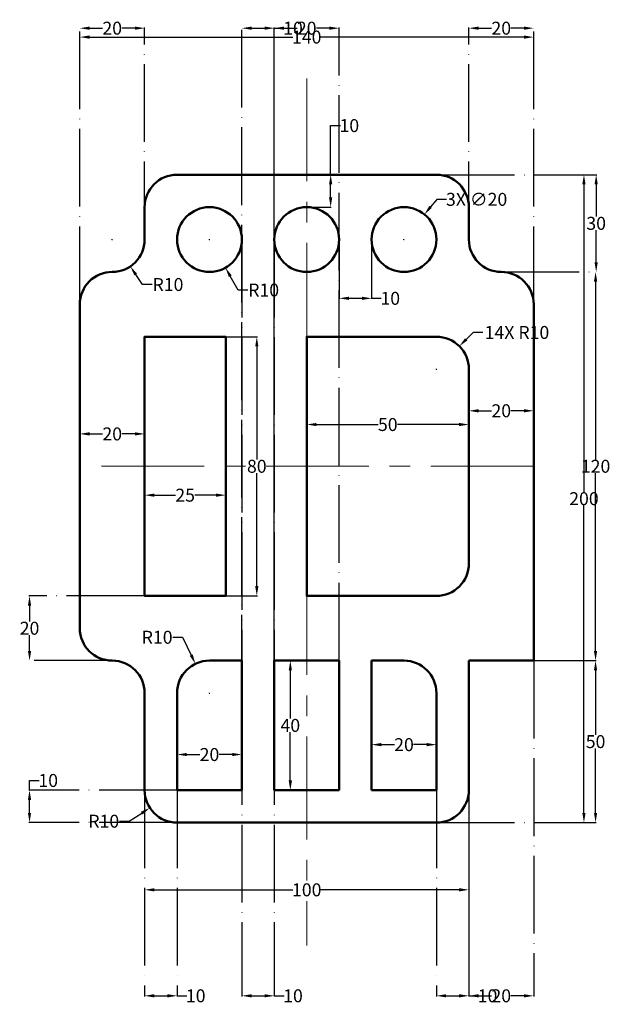
# Model space of a CAD drawing. Units: inches. Extents: x 184 to 366, y 103 to 407.
import ezdxf

# ---------------------------------------------------------------- set-up
doc = ezdxf.new("R2010")
doc.units = ezdxf.units.IN
doc.header["$MEASUREMENT"] = 0
doc.linetypes.add('ACAD_ISO04W100', pattern=[30, 24, -3, 0, -3])
doc.linetypes.add('CENTER', pattern=[50.8, 31.75, -6.35, 6.35, -6.35])
for name, color, linetype, lineweight in [('M-CNTR', 4, 'CENTER', 18), ('M-DIMS', 2, 'Continuous', 25), ('M-OUTL', 7, 'Continuous', 50)]:
    doc.layers.add(name, color=color, linetype=linetype, lineweight=lineweight)
doc.styles.get("Standard").update_dxf_attribs({"font": 'arial.ttf'})
doc.dimstyles.get("Standard").update_dxf_attribs({"dimtxt": 4, "dimasz": 3, "dimexe": 0.18, "dimexo": 0.0625, "dimgap": 0.09, "dimtad": 0, "dimtih": 1, "dimtoh": 1, "dimdec": 0, "dimzin": 0, "dimdsep": 46, "dimtxsty": 'Standard', "dimcen": 0.09, "dimadec": 0, "dimazin": 0, "dimtfac": 1, "dimtdec": 0, "dimtofl": 0, "dimtmove": 0, "dimatfit": 3, "dimfxl": 1, "dimtolj": 1, "dimtzin": 0, "dimarcsym": 0})

# ---------------------------------------------------------------- blocks, each defined once
blk = doc.blocks.new('*D1')
at = {"layer": 'Defpoints', "color": 0, "transparency": 16777216}
for p in [(267.46, 209.15), (267.46, 169.15), (267.46, 169.15)]:
    blk.add_point(p, dxfattribs=at)
at = {"layer": 'M-DIMS', "color": 0, "linetype": 'ACAD_ISO04W100', "lineweight": -2, "transparency": 16777216}
for p, q in [((267.53, 209.15), (267.64, 209.15)), ((267.53, 169.15), (267.64, 169.15))]:
    blk.add_line(p, q, dxfattribs=at)
at = {"layer": 'M-DIMS', "color": 0, "lineweight": -2, "transparency": 16777216}
for p, q in [((267.46, 206.15), (267.46, 191.28)), ((267.46, 172.15), (267.46, 187.02))]:
    blk.add_line(p, q, dxfattribs=at)
at = {"layer": 'M-DIMS', "color": 0, "transparency": 16777216}
for points in [[(266.96, 206.15), (267.96, 206.15), (267.46, 209.15)], [(266.96, 172.15), (267.96, 172.15), (267.46, 169.15)]]:
    blk.add_solid(points, dxfattribs=at)
at = {"layer": 'M-DIMS', "color": 0, "transparency": 16777216, "insert": (267.46, 189.15), "char_height": 4, "attachment_point": 5}
blk.add_mtext('\\A1;40', dxfattribs=at)
blk = doc.blocks.new('*D2')
at = {"layer": 'Defpoints', "color": 0, "transparency": 16777216}
for p in [(232.52, 180.16), (232.52, 180.16), (252.52, 180.16)]:
    blk.add_point(p, dxfattribs=at)
at = {"layer": 'M-DIMS', "color": 0, "linetype": 'ACAD_ISO04W100', "lineweight": -2, "transparency": 16777216}
for p, q in [((232.52, 180.22), (232.52, 180.34)), ((252.52, 180.22), (252.52, 180.34))]:
    blk.add_line(p, q, dxfattribs=at)
at = {"layer": 'M-DIMS', "color": 0, "lineweight": -2, "transparency": 16777216}
for p, q in [((235.52, 180.16), (239.54, 180.16)), ((249.52, 180.16), (245.5, 180.16))]:
    blk.add_line(p, q, dxfattribs=at)
at = {"layer": 'M-DIMS', "color": 0, "transparency": 16777216}
for points in [[(235.52, 180.66), (235.52, 179.66), (232.52, 180.16)], [(249.52, 180.66), (249.52, 179.66), (252.52, 180.16)]]:
    blk.add_solid(points, dxfattribs=at)
at = {"layer": 'M-DIMS', "color": 0, "transparency": 16777216, "insert": (242.52, 180.16), "char_height": 4, "attachment_point": 5}
blk.add_mtext('\\A1;20', dxfattribs=at)
blk = doc.blocks.new('*D3')
at = {"layer": 'Defpoints', "color": 0, "transparency": 16777216}
for p in [(292.52, 183.21), (312.52, 183.21), (312.52, 183.21)]:
    blk.add_point(p, dxfattribs=at)
at = {"layer": 'M-DIMS', "color": 0, "linetype": 'ACAD_ISO04W100', "lineweight": -2, "transparency": 16777216}
for p, q in [((292.52, 183.28), (292.52, 183.39)), ((312.52, 183.28), (312.52, 183.39))]:
    blk.add_line(p, q, dxfattribs=at)
at = {"layer": 'M-DIMS', "color": 0, "lineweight": -2, "transparency": 16777216}
for p, q in [((295.52, 183.21), (299.54, 183.21)), ((309.52, 183.21), (305.5, 183.21))]:
    blk.add_line(p, q, dxfattribs=at)
at = {"layer": 'M-DIMS', "color": 0, "transparency": 16777216}
for points in [[(295.52, 183.71), (295.52, 182.71), (292.52, 183.21)], [(309.52, 183.71), (309.52, 182.71), (312.52, 183.21)]]:
    blk.add_solid(points, dxfattribs=at)
at = {"layer": 'M-DIMS', "color": 0, "transparency": 16777216, "insert": (302.52, 183.21), "char_height": 4, "attachment_point": 5}
blk.add_mtext('\\A1;20', dxfattribs=at)
blk = doc.blocks.new('*D4')
at = {"layer": 'Defpoints', "color": 0, "transparency": 16777216}
for p in [(222.52, 169.15), (322.52, 169.15), (322.52, 138.39)]:
    blk.add_point(p, dxfattribs=at)
at = {"layer": 'M-DIMS', "color": 0, "linetype": 'ACAD_ISO04W100', "lineweight": -2, "transparency": 16777216}
for p, q in [((222.52, 169.09), (222.52, 138.21)), ((322.52, 169.09), (322.52, 138.21))]:
    blk.add_line(p, q, dxfattribs=at)
at = {"layer": 'M-DIMS', "color": 0, "lineweight": -2, "transparency": 16777216}
for p, q in [((225.52, 138.39), (268.2, 138.39)), ((319.52, 138.39), (276.83, 138.39))]:
    blk.add_line(p, q, dxfattribs=at)
at = {"layer": 'M-DIMS', "color": 0, "transparency": 16777216}
for points in [[(225.52, 138.89), (225.52, 137.89), (222.52, 138.39)], [(319.52, 138.89), (319.52, 137.89), (322.52, 138.39)]]:
    blk.add_solid(points, dxfattribs=at)
at = {"layer": 'M-DIMS', "color": 0, "transparency": 16777216, "insert": (272.52, 138.39), "char_height": 4, "attachment_point": 5}
blk.add_mtext('\\A1;100', dxfattribs=at)
blk = doc.blocks.new('*D5')
at = {"layer": 'Defpoints', "color": 0, "transparency": 16777216}
for p in [(272.52, 282.04), (272.52, 269.15), (322.52, 269.15)]:
    blk.add_point(p, dxfattribs=at)
at = {"layer": 'M-DIMS', "color": 0, "linetype": 'ACAD_ISO04W100', "lineweight": -2, "transparency": 16777216}
for p, q in [((272.52, 269.21), (272.52, 282.22)), ((322.52, 269.21), (322.52, 282.22))]:
    blk.add_line(p, q, dxfattribs=at)
at = {"layer": 'M-DIMS', "color": 0, "lineweight": -2, "transparency": 16777216}
for p, q in [((275.52, 282.04), (294.57, 282.04)), ((319.52, 282.04), (300.47, 282.04))]:
    blk.add_line(p, q, dxfattribs=at)
at = {"layer": 'M-DIMS', "color": 0, "transparency": 16777216}
for points in [[(275.52, 282.54), (275.52, 281.54), (272.52, 282.04)], [(319.52, 282.54), (319.52, 281.54), (322.52, 282.04)]]:
    blk.add_solid(points, dxfattribs=at)
at = {"layer": 'M-DIMS', "color": 0, "transparency": 16777216, "insert": (297.52, 282.04), "char_height": 4, "attachment_point": 5}
blk.add_mtext('\\A1;50', dxfattribs=at)
blk = doc.blocks.new('*D6')
at = {"layer": 'Defpoints', "color": 0, "transparency": 16777216}
for p in [(222.52, 269.15), (247.52, 269.15), (222.52, 260.23)]:
    blk.add_point(p, dxfattribs=at)
at = {"layer": 'M-DIMS', "color": 0, "linetype": 'ACAD_ISO04W100', "lineweight": -2, "transparency": 16777216}
for p, q in [((222.52, 269.09), (222.52, 260.05)), ((247.52, 269.09), (247.52, 260.05))]:
    blk.add_line(p, q, dxfattribs=at)
at = {"layer": 'M-DIMS', "color": 0, "lineweight": -2, "transparency": 16777216}
for p, q in [((225.52, 260.23), (232.01, 260.23)), ((244.52, 260.23), (238.02, 260.23))]:
    blk.add_line(p, q, dxfattribs=at)
at = {"layer": 'M-DIMS', "color": 0, "transparency": 16777216}
for points in [[(225.52, 260.73), (225.52, 259.73), (222.52, 260.23)], [(244.52, 260.73), (244.52, 259.73), (247.52, 260.23)]]:
    blk.add_solid(points, dxfattribs=at)
at = {"layer": 'M-DIMS', "color": 0, "transparency": 16777216, "insert": (235.02, 260.23), "char_height": 4, "attachment_point": 5}
blk.add_mtext('\\A1;25', dxfattribs=at)
blk = doc.blocks.new('*D7')
at = {"layer": 'Defpoints', "color": 0, "transparency": 16777216}
for p in [(247.52, 309.15), (247.52, 229.15), (257.12, 229.15)]:
    blk.add_point(p, dxfattribs=at)
at = {"layer": 'M-DIMS', "color": 0, "linetype": 'ACAD_ISO04W100', "lineweight": -2, "transparency": 16777216}
for p, q in [((247.58, 309.15), (257.3, 309.15)), ((247.58, 229.15), (257.3, 229.15))]:
    blk.add_line(p, q, dxfattribs=at)
at = {"layer": 'M-DIMS', "color": 0, "lineweight": -2, "transparency": 16777216}
for p, q in [((257.12, 306.15), (257.12, 271.28)), ((257.12, 232.15), (257.12, 267.02))]:
    blk.add_line(p, q, dxfattribs=at)
at = {"layer": 'M-DIMS', "color": 0, "transparency": 16777216}
for points in [[(256.62, 306.15), (257.62, 306.15), (257.12, 309.15)], [(256.62, 232.15), (257.62, 232.15), (257.12, 229.15)]]:
    blk.add_solid(points, dxfattribs=at)
at = {"layer": 'M-DIMS', "color": 0, "transparency": 16777216, "insert": (257.12, 269.15), "char_height": 4, "attachment_point": 5}
blk.add_mtext('\\A1;80', dxfattribs=at)
blk = doc.blocks.new('*D8')
at = {"layer": 'Defpoints', "color": 0, "transparency": 16777216}
for p in [(202.52, 279.15), (202.52, 279.15), (222.52, 279.15)]:
    blk.add_point(p, dxfattribs=at)
at = {"layer": 'M-DIMS', "color": 0, "linetype": 'ACAD_ISO04W100', "lineweight": -2, "transparency": 16777216}
for p, q in [((202.52, 279.22), (202.52, 279.33)), ((222.52, 279.22), (222.52, 279.33))]:
    blk.add_line(p, q, dxfattribs=at)
at = {"layer": 'M-DIMS', "color": 0, "lineweight": -2, "transparency": 16777216}
for p, q in [((205.52, 279.15), (209.54, 279.15)), ((219.52, 279.15), (215.5, 279.15))]:
    blk.add_line(p, q, dxfattribs=at)
at = {"layer": 'M-DIMS', "color": 0, "transparency": 16777216}
for points in [[(205.52, 279.65), (205.52, 278.65), (202.52, 279.15)], [(219.52, 279.65), (219.52, 278.65), (222.52, 279.15)]]:
    blk.add_solid(points, dxfattribs=at)
at = {"layer": 'M-DIMS', "color": 0, "transparency": 16777216, "insert": (212.52, 279.15), "char_height": 4, "attachment_point": 5}
blk.add_mtext('\\A1;20', dxfattribs=at)
blk = doc.blocks.new('*D9')
at = {"layer": 'Defpoints', "color": 0, "transparency": 16777216}
for p in [(322.52, 286.28), (342.52, 286.28), (342.52, 286.28)]:
    blk.add_point(p, dxfattribs=at)
at = {"layer": 'M-DIMS', "color": 0, "linetype": 'ACAD_ISO04W100', "lineweight": -2, "transparency": 16777216}
for p, q in [((322.52, 286.35), (322.52, 286.46)), ((342.52, 286.35), (342.52, 286.46))]:
    blk.add_line(p, q, dxfattribs=at)
at = {"layer": 'M-DIMS', "color": 0, "lineweight": -2, "transparency": 16777216}
for p, q in [((325.52, 286.28), (329.54, 286.28)), ((339.52, 286.28), (335.5, 286.28))]:
    blk.add_line(p, q, dxfattribs=at)
at = {"layer": 'M-DIMS', "color": 0, "transparency": 16777216}
for points in [[(325.52, 286.78), (325.52, 285.78), (322.52, 286.28)], [(339.52, 286.78), (339.52, 285.78), (342.52, 286.28)]]:
    blk.add_solid(points, dxfattribs=at)
at = {"layer": 'M-DIMS', "color": 0, "transparency": 16777216, "insert": (332.52, 286.28), "char_height": 4, "attachment_point": 5}
blk.add_mtext('\\A1;20', dxfattribs=at)
blk = doc.blocks.new('*D10')
at = {"layer": 'Defpoints', "color": 0, "transparency": 16777216}
for p in [(272.52, 359.15), (279.9, 359.15), (272.52, 349.15)]:
    blk.add_point(p, dxfattribs=at)
at = {"layer": 'M-DIMS', "color": 0, "lineweight": -2, "transparency": 16777216}
for p, q in [((279.9, 359.15), (279.9, 374.33)), ((279.9, 374.33), (282.9, 374.33)), ((279.9, 352.15), (279.9, 356.15))]:
    blk.add_line(p, q, dxfattribs=at)
at = {"layer": 'M-DIMS', "color": 0, "linetype": 'ACAD_ISO04W100', "lineweight": -2, "transparency": 16777216}
for p, q in [((272.58, 359.15), (280.08, 359.15)), ((272.58, 349.15), (280.08, 349.15))]:
    blk.add_line(p, q, dxfattribs=at)
at = {"layer": 'M-DIMS', "color": 0, "transparency": 16777216}
for points in [[(279.4, 356.15), (280.4, 356.15), (279.9, 359.15)], [(279.4, 352.15), (280.4, 352.15), (279.9, 349.15)]]:
    blk.add_solid(points, dxfattribs=at)
at = {"layer": 'M-DIMS', "color": 0, "transparency": 16777216, "insert": (285.66, 374.33), "char_height": 4, "attachment_point": 5}
blk.add_mtext('\\A1;10', dxfattribs=at)
blk = doc.blocks.new('*D11')
at = {"layer": 'Defpoints', "color": 0, "transparency": 16777216}
for p in [(282.52, 339.15), (292.52, 339.15), (292.52, 321)]:
    blk.add_point(p, dxfattribs=at)
at = {"layer": 'M-DIMS', "color": 0, "linetype": 'ACAD_ISO04W100', "lineweight": -2, "transparency": 16777216}
for p, q in [((282.52, 339.09), (282.52, 320.82)), ((292.52, 339.09), (292.52, 320.82))]:
    blk.add_line(p, q, dxfattribs=at)
at = {"layer": 'M-DIMS', "color": 0, "lineweight": -2, "transparency": 16777216}
for p, q in [((285.52, 321), (289.52, 321)), ((292.52, 321), (295.52, 321))]:
    blk.add_line(p, q, dxfattribs=at)
at = {"layer": 'M-DIMS', "color": 0, "transparency": 16777216}
for points in [[(285.52, 321.5), (285.52, 320.5), (282.52, 321)], [(289.52, 321.5), (289.52, 320.5), (292.52, 321)]]:
    blk.add_solid(points, dxfattribs=at)
at = {"layer": 'M-DIMS', "color": 0, "transparency": 16777216, "insert": (298.28, 321), "char_height": 4, "attachment_point": 5}
blk.add_mtext('\\A1;10', dxfattribs=at)
blk = doc.blocks.new('*D12')
at = {"layer": 'Defpoints', "color": 0, "transparency": 16777216}
for p in [(242.52, 339.15), (247.45, 330.45)]:
    blk.add_point(p, dxfattribs=at)
at = {"layer": 'M-DIMS', "color": 0, "lineweight": -2, "transparency": 16777216}
for p, q in [((242.43, 339.15), (242.61, 339.15)), ((242.52, 339.06), (242.52, 339.24)), ((251.36, 323.56), (248.93, 327.84)), ((254.36, 323.56), (251.36, 323.56))]:
    blk.add_line(p, q, dxfattribs=at)
at = {"layer": 'M-DIMS', "color": 0, "transparency": 16777216}
blk.add_solid([(249.37, 328.09), (248.5, 327.6), (247.45, 330.45)], dxfattribs=at)
at = {"layer": 'M-DIMS', "color": 0, "transparency": 16777216, "insert": (259.23, 323.56), "char_height": 4, "attachment_point": 5}
blk.add_mtext('\\A1;R10', dxfattribs=at)
blk = doc.blocks.new('*D13')
at = {"layer": 'Defpoints', "color": 0, "transparency": 16777216}
for p in [(212.52, 339.15), (218.1, 330.85)]:
    blk.add_point(p, dxfattribs=at)
at = {"layer": 'M-DIMS', "color": 0, "lineweight": -2, "transparency": 16777216}
for p, q in [((212.43, 339.15), (212.61, 339.15)), ((212.52, 339.06), (212.52, 339.24)), ((221.85, 325.26), (219.77, 328.36)), ((224.85, 325.26), (221.85, 325.26))]:
    blk.add_line(p, q, dxfattribs=at)
at = {"layer": 'M-DIMS', "color": 0, "transparency": 16777216}
blk.add_solid([(220.19, 328.64), (219.36, 328.08), (218.1, 330.85)], dxfattribs=at)
at = {"layer": 'M-DIMS', "color": 0, "transparency": 16777216, "insert": (229.72, 325.26), "char_height": 4, "attachment_point": 5}
blk.add_mtext('\\A1;R10', dxfattribs=at)
blk = doc.blocks.new('*D14')
at = {"layer": 'Defpoints', "color": 0, "transparency": 16777216}
for p in [(238.18, 208.16), (242.52, 199.15)]:
    blk.add_point(p, dxfattribs=at)
at = {"layer": 'M-DIMS', "color": 0, "lineweight": -2, "transparency": 16777216}
for p, q in [((231.24, 216.36), (234.24, 216.36)), ((234.24, 216.36), (236.88, 210.86)), ((242.43, 199.15), (242.61, 199.15)), ((242.52, 199.06), (242.52, 199.24))]:
    blk.add_line(p, q, dxfattribs=at)
at = {"layer": 'M-DIMS', "color": 0, "transparency": 16777216}
blk.add_solid([(237.33, 211.08), (236.43, 210.65), (238.18, 208.16)], dxfattribs=at)
at = {"layer": 'M-DIMS', "color": 0, "transparency": 16777216, "insert": (226.38, 216.36), "char_height": 4, "attachment_point": 5}
blk.add_mtext('\\A1;R10', dxfattribs=at)
blk = doc.blocks.new('*D15')
at = {"layer": 'Defpoints', "color": 0, "transparency": 16777216}
for p in [(232.52, 169.15), (224.13, 163.7)]:
    blk.add_point(p, dxfattribs=at)
at = {"layer": 'M-DIMS', "color": 0, "lineweight": -2, "transparency": 16777216}
for p, q in [((232.43, 169.15), (232.61, 169.15)), ((232.52, 169.06), (232.52, 169.24)), ((217.77, 159.57), (221.62, 162.07)), ((214.77, 159.57), (217.77, 159.57))]:
    blk.add_line(p, q, dxfattribs=at)
at = {"layer": 'M-DIMS', "color": 0, "transparency": 16777216}
blk.add_solid([(221.34, 162.49), (221.89, 161.65), (224.13, 163.7)], dxfattribs=at)
at = {"layer": 'M-DIMS', "color": 0, "transparency": 16777216, "insert": (209.91, 159.57), "char_height": 4, "attachment_point": 5}
blk.add_mtext('\\A1;R10', dxfattribs=at)
blk = doc.blocks.new('*D16')
at = {"layer": 'Defpoints', "color": 0, "transparency": 16777216}
for p in [(342.52, 209.15), (312.52, 159.15), (361.61, 159.15)]:
    blk.add_point(p, dxfattribs=at)
at = {"layer": 'M-DIMS', "color": 0, "linetype": 'ACAD_ISO04W100', "lineweight": -2, "transparency": 16777216}
for p, q in [((342.58, 209.15), (361.79, 209.15)), ((312.58, 159.15), (361.79, 159.15))]:
    blk.add_line(p, q, dxfattribs=at)
at = {"layer": 'M-DIMS', "color": 0, "lineweight": -2, "transparency": 16777216}
for p, q in [((361.61, 206.15), (361.61, 186.28)), ((361.61, 162.15), (361.61, 182.02))]:
    blk.add_line(p, q, dxfattribs=at)
at = {"layer": 'M-DIMS', "color": 0, "transparency": 16777216}
for points in [[(361.11, 206.15), (362.11, 206.15), (361.61, 209.15)], [(361.11, 162.15), (362.11, 162.15), (361.61, 159.15)]]:
    blk.add_solid(points, dxfattribs=at)
at = {"layer": 'M-DIMS', "color": 0, "transparency": 16777216, "insert": (361.61, 184.15), "char_height": 4, "attachment_point": 5}
blk.add_mtext('\\A1;50', dxfattribs=at)
blk = doc.blocks.new('*D17')
at = {"layer": 'Defpoints', "color": 0, "transparency": 16777216}
for p in [(332.52, 329.15), (342.52, 209.15), (361.61, 209.15)]:
    blk.add_point(p, dxfattribs=at)
at = {"layer": 'M-DIMS', "color": 0, "linetype": 'ACAD_ISO04W100', "lineweight": -2, "transparency": 16777216}
for p, q in [((332.58, 329.15), (361.79, 329.15)), ((342.58, 209.15), (361.79, 209.15))]:
    blk.add_line(p, q, dxfattribs=at)
at = {"layer": 'M-DIMS', "color": 0, "lineweight": -2, "transparency": 16777216}
for p, q in [((361.61, 326.15), (361.61, 271.28)), ((361.61, 212.15), (361.61, 267.02))]:
    blk.add_line(p, q, dxfattribs=at)
at = {"layer": 'M-DIMS', "color": 0, "transparency": 16777216}
for points in [[(361.11, 326.15), (362.11, 326.15), (361.61, 329.15)], [(361.11, 212.15), (362.11, 212.15), (361.61, 209.15)]]:
    blk.add_solid(points, dxfattribs=at)
at = {"layer": 'M-DIMS', "color": 0, "transparency": 16777216, "insert": (361.61, 269.15), "char_height": 4, "attachment_point": 5}
blk.add_mtext('\\A1;120', dxfattribs=at)
blk = doc.blocks.new('*D18')
at = {"layer": 'Defpoints', "color": 0, "transparency": 16777216}
for p in [(312.52, 359.15), (332.52, 329.15), (361.79, 329.15)]:
    blk.add_point(p, dxfattribs=at)
at = {"layer": 'M-DIMS', "color": 0, "linetype": 'ACAD_ISO04W100', "lineweight": -2, "transparency": 16777216}
for p, q in [((312.58, 359.15), (361.97, 359.15)), ((332.58, 329.15), (361.97, 329.15))]:
    blk.add_line(p, q, dxfattribs=at)
at = {"layer": 'M-DIMS', "color": 0, "lineweight": -2, "transparency": 16777216}
for p, q in [((361.79, 356.15), (361.79, 346.28)), ((361.79, 332.15), (361.79, 342.02))]:
    blk.add_line(p, q, dxfattribs=at)
at = {"layer": 'M-DIMS', "color": 0, "transparency": 16777216}
for points in [[(361.29, 356.15), (362.29, 356.15), (361.79, 359.15)], [(361.29, 332.15), (362.29, 332.15), (361.79, 329.15)]]:
    blk.add_solid(points, dxfattribs=at)
at = {"layer": 'M-DIMS', "color": 0, "transparency": 16777216, "insert": (361.79, 344.15), "char_height": 4, "attachment_point": 5}
blk.add_mtext('\\A1;30', dxfattribs=at)
blk = doc.blocks.new('*D19')
at = {"layer": 'Defpoints', "color": 0, "transparency": 16777216}
for p in [(342.52, 401.65), (202.52, 319.15), (342.52, 319.15)]:
    blk.add_point(p, dxfattribs=at)
at = {"layer": 'M-DIMS', "color": 0, "linetype": 'ACAD_ISO04W100', "lineweight": -2, "transparency": 16777216}
for p, q in [((202.52, 319.21), (202.52, 401.83)), ((342.52, 319.21), (342.52, 401.83))]:
    blk.add_line(p, q, dxfattribs=at)
at = {"layer": 'M-DIMS', "color": 0, "lineweight": -2, "transparency": 16777216}
for p, q in [((205.52, 401.65), (268.2, 401.65)), ((339.52, 401.65), (276.83, 401.65))]:
    blk.add_line(p, q, dxfattribs=at)
at = {"layer": 'M-DIMS', "color": 0, "transparency": 16777216}
for points in [[(205.52, 402.15), (205.52, 401.15), (202.52, 401.65)], [(339.52, 402.15), (339.52, 401.15), (342.52, 401.65)]]:
    blk.add_solid(points, dxfattribs=at)
at = {"layer": 'M-DIMS', "color": 0, "transparency": 16777216, "insert": (272.52, 401.65), "char_height": 4, "attachment_point": 5}
blk.add_mtext('\\A1;140', dxfattribs=at)
blk = doc.blocks.new('SLOT-CORNER-R10')
for p, q in [((0, 0), (0, 40)), ((0, 40), (10, 40)), ((20, 30), (20, 0)), ((20, 0), (0, 0))]:
    blk.add_line(p, q)
blk.add_arc((10, 30), 10, 0, 90)
blk = doc.blocks.new('HOLE-D20')
blk.add_circle((10, 10), 10)
blk = doc.blocks.new('*D22')
at = {"layer": 'Defpoints', "color": 0, "transparency": 16777216}
for p in [(312.52, 359.15), (358.02, 359.15), (312.52, 159.15)]:
    blk.add_point(p, dxfattribs=at)
at = {"layer": 'M-DIMS', "color": 0, "linetype": 'ACAD_ISO04W100', "lineweight": -2, "transparency": 16777216}
for p, q in [((312.58, 359.15), (358.2, 359.15)), ((312.58, 159.15), (358.2, 159.15))]:
    blk.add_line(p, q, dxfattribs=at)
at = {"layer": 'M-DIMS', "color": 0, "lineweight": -2, "transparency": 16777216}
for p, q in [((358.02, 356.15), (358.02, 261.28)), ((358.02, 162.15), (358.02, 257.02))]:
    blk.add_line(p, q, dxfattribs=at)
at = {"layer": 'M-DIMS', "color": 0, "transparency": 16777216}
for points in [[(357.52, 356.15), (358.52, 356.15), (358.02, 359.15)], [(357.52, 162.15), (358.52, 162.15), (358.02, 159.15)]]:
    blk.add_solid(points, dxfattribs=at)
at = {"layer": 'M-DIMS', "color": 0, "transparency": 16777216, "insert": (358.02, 259.15), "char_height": 4, "attachment_point": 5}
blk.add_mtext('\\A1;200', dxfattribs=at)
blk = doc.blocks.new('*D23')
at = {"layer": 'Defpoints', "color": 0, "transparency": 16777216}
for p in [(252.52, 339.15), (262.52, 339.15), (262.52, 105.67)]:
    blk.add_point(p, dxfattribs=at)
at = {"layer": 'M-DIMS', "color": 0, "linetype": 'ACAD_ISO04W100', "lineweight": -2, "transparency": 16777216}
for p, q in [((252.52, 339.09), (252.52, 105.49)), ((262.52, 339.09), (262.52, 105.49))]:
    blk.add_line(p, q, dxfattribs=at)
at = {"layer": 'M-DIMS', "color": 0, "lineweight": -2, "transparency": 16777216}
for p, q in [((255.52, 105.67), (259.52, 105.67)), ((262.52, 105.67), (265.52, 105.67))]:
    blk.add_line(p, q, dxfattribs=at)
at = {"layer": 'M-DIMS', "color": 0, "transparency": 16777216}
for points in [[(255.52, 106.17), (255.52, 105.17), (252.52, 105.67)], [(259.52, 106.17), (259.52, 105.17), (262.52, 105.67)]]:
    blk.add_solid(points, dxfattribs=at)
at = {"layer": 'M-DIMS', "color": 0, "transparency": 16777216, "insert": (268.28, 105.67), "char_height": 4, "attachment_point": 5}
blk.add_mtext('\\A1;10', dxfattribs=at)
blk = doc.blocks.new('*D24')
at = {"layer": 'Defpoints', "color": 0, "transparency": 16777216}
for p in [(222.52, 169.15), (232.52, 169.15), (232.52, 105.67)]:
    blk.add_point(p, dxfattribs=at)
at = {"layer": 'M-DIMS', "color": 0, "linetype": 'ACAD_ISO04W100', "lineweight": -2, "transparency": 16777216}
for p, q in [((222.52, 169.09), (222.52, 105.49)), ((232.52, 169.09), (232.52, 105.49))]:
    blk.add_line(p, q, dxfattribs=at)
at = {"layer": 'M-DIMS', "color": 0, "lineweight": -2, "transparency": 16777216}
for p, q in [((225.52, 105.67), (229.52, 105.67)), ((232.52, 105.67), (235.52, 105.67))]:
    blk.add_line(p, q, dxfattribs=at)
at = {"layer": 'M-DIMS', "color": 0, "transparency": 16777216}
for points in [[(225.52, 106.17), (225.52, 105.17), (222.52, 105.67)], [(229.52, 106.17), (229.52, 105.17), (232.52, 105.67)]]:
    blk.add_solid(points, dxfattribs=at)
at = {"layer": 'M-DIMS', "color": 0, "transparency": 16777216, "insert": (238.28, 105.67), "char_height": 4, "attachment_point": 5}
blk.add_mtext('\\A1;10', dxfattribs=at)
blk = doc.blocks.new('*D25')
at = {"layer": 'Defpoints', "color": 0, "transparency": 16777216}
for p in [(262.52, 404.4), (252.52, 169.15), (262.52, 169.15)]:
    blk.add_point(p, dxfattribs=at)
at = {"layer": 'M-DIMS', "color": 0, "linetype": 'ACAD_ISO04W100', "lineweight": -2, "transparency": 16777216}
for p, q in [((252.52, 169.21), (252.52, 404.58)), ((262.52, 169.21), (262.52, 404.58))]:
    blk.add_line(p, q, dxfattribs=at)
at = {"layer": 'M-DIMS', "color": 0, "lineweight": -2, "transparency": 16777216}
for p, q in [((255.52, 404.4), (259.52, 404.4)), ((262.52, 404.4), (265.52, 404.4))]:
    blk.add_line(p, q, dxfattribs=at)
at = {"layer": 'M-DIMS', "color": 0, "transparency": 16777216}
for points in [[(255.52, 404.9), (255.52, 403.9), (252.52, 404.4)], [(259.52, 404.9), (259.52, 403.9), (262.52, 404.4)]]:
    blk.add_solid(points, dxfattribs=at)
at = {"layer": 'M-DIMS', "color": 0, "transparency": 16777216, "insert": (268.28, 404.4), "char_height": 4, "attachment_point": 5}
blk.add_mtext('\\A1;10', dxfattribs=at)
blk = doc.blocks.new('*D26')
at = {"layer": 'Defpoints', "color": 0, "transparency": 16777216}
for p in [(187.02, 169.15), (232.52, 169.15), (232.52, 159.15)]:
    blk.add_point(p, dxfattribs=at)
at = {"layer": 'M-DIMS', "color": 0, "lineweight": -2, "transparency": 16777216}
for p, q in [((187.02, 169.15), (187.02, 172.15)), ((187.02, 172.15), (190.02, 172.15)), ((187.02, 162.15), (187.02, 166.15))]:
    blk.add_line(p, q, dxfattribs=at)
at = {"layer": 'M-DIMS', "color": 0, "linetype": 'ACAD_ISO04W100', "lineweight": -2, "transparency": 16777216}
for p, q in [((232.45, 169.15), (186.84, 169.15)), ((232.45, 159.15), (186.84, 159.15))]:
    blk.add_line(p, q, dxfattribs=at)
at = {"layer": 'M-DIMS', "color": 0, "transparency": 16777216}
for points in [[(186.52, 166.15), (187.52, 166.15), (187.02, 169.15)], [(186.52, 162.15), (187.52, 162.15), (187.02, 159.15)]]:
    blk.add_solid(points, dxfattribs=at)
at = {"layer": 'M-DIMS', "color": 0, "transparency": 16777216, "insert": (192.78, 172.15), "char_height": 4, "attachment_point": 5}
blk.add_mtext('\\A1;10', dxfattribs=at)
blk = doc.blocks.new('*D27')
at = {"layer": 'Defpoints', "color": 0, "transparency": 16777216}
for p in [(187.02, 229.15), (222.52, 229.15), (212.52, 209.15)]:
    blk.add_point(p, dxfattribs=at)
at = {"layer": 'M-DIMS', "color": 0, "linetype": 'ACAD_ISO04W100', "lineweight": -2, "transparency": 16777216}
for p, q in [((222.45, 229.15), (186.84, 229.15)), ((212.45, 209.15), (186.84, 209.15))]:
    blk.add_line(p, q, dxfattribs=at)
at = {"layer": 'M-DIMS', "color": 0, "lineweight": -2, "transparency": 16777216}
for p, q in [((187.02, 226.15), (187.02, 221.28)), ((187.02, 212.15), (187.02, 217.02))]:
    blk.add_line(p, q, dxfattribs=at)
at = {"layer": 'M-DIMS', "color": 0, "transparency": 16777216}
for points in [[(186.52, 226.15), (187.52, 226.15), (187.02, 229.15)], [(186.52, 212.15), (187.52, 212.15), (187.02, 209.15)]]:
    blk.add_solid(points, dxfattribs=at)
at = {"layer": 'M-DIMS', "color": 0, "transparency": 16777216, "insert": (187.02, 219.15), "char_height": 4, "attachment_point": 5}
blk.add_mtext('\\A1;20', dxfattribs=at)
blk = doc.blocks.new('*D28')
at = {"layer": 'Defpoints', "color": 0, "transparency": 16777216}
for p in [(342.52, 404.4), (322.52, 339.15), (342.52, 319.15)]:
    blk.add_point(p, dxfattribs=at)
at = {"layer": 'M-DIMS', "color": 0, "linetype": 'ACAD_ISO04W100', "lineweight": -2, "transparency": 16777216}
for p, q in [((322.52, 339.21), (322.52, 404.58)), ((342.52, 319.21), (342.52, 404.58))]:
    blk.add_line(p, q, dxfattribs=at)
at = {"layer": 'M-DIMS', "color": 0, "lineweight": -2, "transparency": 16777216}
for p, q in [((325.52, 404.4), (329.54, 404.4)), ((339.52, 404.4), (335.5, 404.4))]:
    blk.add_line(p, q, dxfattribs=at)
at = {"layer": 'M-DIMS', "color": 0, "transparency": 16777216}
for points in [[(325.52, 404.9), (325.52, 403.9), (322.52, 404.4)], [(339.52, 404.9), (339.52, 403.9), (342.52, 404.4)]]:
    blk.add_solid(points, dxfattribs=at)
at = {"layer": 'M-DIMS', "color": 0, "transparency": 16777216, "insert": (332.52, 404.4), "char_height": 4, "attachment_point": 5}
blk.add_mtext('\\A1;20', dxfattribs=at)
blk = doc.blocks.new('*D29')
at = {"layer": 'Defpoints', "color": 0, "transparency": 16777216}
for p in [(322.52, 209.15), (342.52, 209.15), (342.52, 105.67)]:
    blk.add_point(p, dxfattribs=at)
at = {"layer": 'M-DIMS', "color": 0, "linetype": 'ACAD_ISO04W100', "lineweight": -2, "transparency": 16777216}
for p, q in [((322.52, 209.09), (322.52, 105.49)), ((342.52, 209.09), (342.52, 105.49))]:
    blk.add_line(p, q, dxfattribs=at)
at = {"layer": 'M-DIMS', "color": 0, "lineweight": -2, "transparency": 16777216}
for p, q in [((325.52, 105.67), (329.54, 105.67)), ((339.52, 105.67), (335.5, 105.67))]:
    blk.add_line(p, q, dxfattribs=at)
at = {"layer": 'M-DIMS', "color": 0, "transparency": 16777216}
for points in [[(325.52, 106.17), (325.52, 105.17), (322.52, 105.67)], [(339.52, 106.17), (339.52, 105.17), (342.52, 105.67)]]:
    blk.add_solid(points, dxfattribs=at)
at = {"layer": 'M-DIMS', "color": 0, "transparency": 16777216, "insert": (332.52, 105.67), "char_height": 4, "attachment_point": 5}
blk.add_mtext('\\A1;20', dxfattribs=at)
blk = doc.blocks.new('*D30')
at = {"layer": 'Defpoints', "color": 0, "transparency": 16777216}
for p in [(282.52, 404.4), (262.52, 209.15), (282.52, 209.15)]:
    blk.add_point(p, dxfattribs=at)
at = {"layer": 'M-DIMS', "color": 0, "linetype": 'ACAD_ISO04W100', "lineweight": -2, "transparency": 16777216}
for p, q in [((262.52, 209.21), (262.52, 404.58)), ((282.52, 209.21), (282.52, 404.58))]:
    blk.add_line(p, q, dxfattribs=at)
at = {"layer": 'M-DIMS', "color": 0, "lineweight": -2, "transparency": 16777216}
for p, q in [((265.52, 404.4), (269.54, 404.4)), ((279.52, 404.4), (275.5, 404.4))]:
    blk.add_line(p, q, dxfattribs=at)
at = {"layer": 'M-DIMS', "color": 0, "transparency": 16777216}
for points in [[(265.52, 404.9), (265.52, 403.9), (262.52, 404.4)], [(279.52, 404.9), (279.52, 403.9), (282.52, 404.4)]]:
    blk.add_solid(points, dxfattribs=at)
at = {"layer": 'M-DIMS', "color": 0, "transparency": 16777216, "insert": (272.52, 404.4), "char_height": 4, "attachment_point": 5}
blk.add_mtext('\\A1;20', dxfattribs=at)
blk = doc.blocks.new('*D31')
at = {"layer": 'Defpoints', "color": 0, "transparency": 16777216}
for p in [(222.52, 404.4), (222.52, 339.15), (202.52, 319.15)]:
    blk.add_point(p, dxfattribs=at)
at = {"layer": 'M-DIMS', "color": 0, "linetype": 'ACAD_ISO04W100', "lineweight": -2, "transparency": 16777216}
for p, q in [((202.52, 319.21), (202.52, 404.58)), ((222.52, 339.21), (222.52, 404.58))]:
    blk.add_line(p, q, dxfattribs=at)
at = {"layer": 'M-DIMS', "color": 0, "lineweight": -2, "transparency": 16777216}
for p, q in [((205.52, 404.4), (209.54, 404.4)), ((219.52, 404.4), (215.5, 404.4))]:
    blk.add_line(p, q, dxfattribs=at)
at = {"layer": 'M-DIMS', "color": 0, "transparency": 16777216}
for points in [[(205.52, 404.9), (205.52, 403.9), (202.52, 404.4)], [(219.52, 404.9), (219.52, 403.9), (222.52, 404.4)]]:
    blk.add_solid(points, dxfattribs=at)
at = {"layer": 'M-DIMS', "color": 0, "transparency": 16777216, "insert": (212.52, 404.4), "char_height": 4, "attachment_point": 5}
blk.add_mtext('\\A1;20', dxfattribs=at)
blk = doc.blocks.new('*D32')
at = {"layer": 'Defpoints', "color": 0, "transparency": 16777216}
for p in [(312.52, 169.15), (322.52, 169.15), (322.52, 105.67)]:
    blk.add_point(p, dxfattribs=at)
at = {"layer": 'M-DIMS', "color": 0, "linetype": 'ACAD_ISO04W100', "lineweight": -2, "transparency": 16777216}
for p, q in [((312.52, 169.09), (312.52, 105.49)), ((322.52, 169.09), (322.52, 105.49))]:
    blk.add_line(p, q, dxfattribs=at)
at = {"layer": 'M-DIMS', "color": 0, "lineweight": -2, "transparency": 16777216}
for p, q in [((315.52, 105.67), (319.52, 105.67)), ((322.52, 105.67), (325.52, 105.67))]:
    blk.add_line(p, q, dxfattribs=at)
at = {"layer": 'M-DIMS', "color": 0, "transparency": 16777216}
for points in [[(315.52, 106.17), (315.52, 105.17), (312.52, 105.67)], [(319.52, 106.17), (319.52, 105.17), (322.52, 105.67)]]:
    blk.add_solid(points, dxfattribs=at)
at = {"layer": 'M-DIMS', "color": 0, "transparency": 16777216, "insert": (328.28, 105.67), "char_height": 4, "attachment_point": 5}
blk.add_mtext('\\A1;10', dxfattribs=at)
blk = doc.blocks.new('*D33')
at = {"layer": 'Defpoints', "color": 0, "transparency": 16777216}
for p in [(319.59, 306.22), (312.52, 299.15)]:
    blk.add_point(p, dxfattribs=at)
at = {"layer": 'M-DIMS', "color": 0, "lineweight": -2, "transparency": 16777216}
for p, q in [((323.83, 310.46), (321.71, 308.34)), ((326.83, 310.46), (323.83, 310.46)), ((312.43, 299.15), (312.61, 299.15)), ((312.52, 299.06), (312.52, 299.24))]:
    blk.add_line(p, q, dxfattribs=at)
at = {"layer": 'M-DIMS', "color": 0, "transparency": 16777216}
blk.add_solid([(321.36, 308.69), (322.06, 307.99), (319.59, 306.22)], dxfattribs=at)
at = {"layer": 'M-DIMS', "color": 0, "transparency": 16777216, "insert": (337.36, 310.46), "char_height": 4, "attachment_point": 5}
blk.add_mtext('\\A1;14X R10', dxfattribs=at)
blk = doc.blocks.new('*D34')
at = {"layer": 'Defpoints', "color": 0, "transparency": 16777216}
for p in [(308.83, 346.91), (296.21, 331.39)]:
    blk.add_point(p, dxfattribs=at)
at = {"layer": 'M-DIMS', "color": 0, "lineweight": -2, "transparency": 16777216}
for p, q in [((312.61, 351.56), (310.72, 349.24)), ((315.61, 351.56), (312.61, 351.56)), ((302.43, 339.15), (302.61, 339.15)), ((302.52, 339.06), (302.52, 339.24))]:
    blk.add_line(p, q, dxfattribs=at)
at = {"layer": 'M-DIMS', "color": 0, "transparency": 16777216}
blk.add_solid([(310.33, 349.55), (311.11, 348.92), (308.83, 346.91)], dxfattribs=at)
at = {"layer": 'M-DIMS', "color": 0, "transparency": 16777216, "insert": (324.92, 351.56), "char_height": 4, "attachment_point": 5}
blk.add_mtext('\\A1;3X ∅20', dxfattribs=at)

msp = doc.modelspace()

# ---------------------------------------------------------------- linework, layer by layer
at = {"layer": 'M-CNTR'}
for p, q in [((272.52, 388.9), (272.52, 121.17)), ((342.52, 269.15), (202.52, 269.15))]:
    msp.add_line(p, q, dxfattribs=at)
at = {"layer": 'M-OUTL'}
for p, q in [((312.52, 359.15), (232.52, 359.15)), ((222.52, 349.15), (222.52, 339.15)), ((322.52, 339.15), (322.52, 349.15)), ((212.52, 329.15), (212.52, 329.15)), ((332.52, 329.15), (332.52, 329.15)), ((202.52, 319.15), (202.52, 219.15)), ((342.52, 209.15), (342.52, 319.15)), ((212.52, 209.15), (212.52, 209.15)), ((262.52, 169.15), (262.52, 209.15)), ((272.52, 209.15), (262.52, 209.15)), ((272.52, 209.15), (282.52, 209.15)), ((282.52, 209.15), (282.52, 169.15)), ((322.52, 169.15), (322.52, 209.15)), ((322.52, 209.15), (342.52, 209.15)), ((332.52, 209.15), (332.52, 209.15)), ((222.52, 199.15), (222.52, 169.15)), ((282.52, 169.15), (262.52, 169.15)), ((232.52, 159.15), (312.52, 159.15))]:
    msp.add_line(p, q, dxfattribs=at)
msp.add_lwpolyline([(222.52, 269.15), (222.52, 309.15), (247.52, 309.15), (247.52, 229.15), (222.52, 229.15)], close=True, dxfattribs=at)
msp.add_lwpolyline([(322.52, 239.15), (322.52, 299.15, 0.414214), (312.52, 309.15), (272.52, 309.15), (272.52, 229.15), (312.52, 229.15, 0.414214)], format="xyb", close=True, dxfattribs=at)
for centre, start, end in [((232.52, 349.15), 90, 180), ((312.52, 349.15), 0, 90), ((212.52, 339.15), 270, 0), ((332.52, 339.15), 180, 270), ((212.52, 319.15), 90, 180), ((332.52, 319.15), 0, 90), ((212.52, 219.15), 180, 270), ((212.52, 199.15), 0, 90), ((232.52, 169.15), 180, 270), ((312.52, 169.15), 270, 0)]:
    msp.add_arc(centre, 10, start, end, dxfattribs=at)

# ---------------------------------------------------------------- block references
for name, p in [('HOLE-D20', (232.52, 329.15)), ('HOLE-D20', (262.52, 329.15)), ('HOLE-D20', (292.52, 329.15)), ('SLOT-CORNER-R10', (292.52, 169.15))]:
    msp.add_blockref(name, p, dxfattribs=at)
at = {"layer": 'M-OUTL', "extrusion": (0, 0, -1), "zscale": -1}
msp.add_blockref('SLOT-CORNER-R10', (-252.52, 169.15), dxfattribs=at)

# ---------------------------------------------------------------- dimensions: what is measured, and where the dimension line sits
at = {"layer": 'M-DIMS'}
for base, p1, p2, override, picture, middle in [((222.52, 404.4), (202.52, 319.15), (222.52, 339.15), {"dimdec": 0, "dimlfac": 1, "dimrnd": 0, "dimzin": 0, "dimdsep": 46, "dimlunit": 2}, '*D31', (212.52, 404.4)), ((262.52, 404.4), (252.52, 169.15), (262.52, 169.15), {"dimdec": 0, "dimlfac": 1, "dimrnd": 0, "dimzin": 0, "dimdsep": 46, "dimlunit": 2}, '*D25', (268.28, 404.4)), ((282.52, 404.4), (262.52, 209.15), (282.52, 209.15), {"dimdec": 0, "dimlfac": 1, "dimrnd": 0, "dimzin": 0, "dimdsep": 46, "dimlunit": 2}, '*D30', (272.52, 404.4)), ((342.52, 404.4), (322.52, 339.15), (342.52, 319.15), {"dimdec": 0, "dimlfac": 1, "dimrnd": 0, "dimzin": 0, "dimdsep": 46, "dimlunit": 2}, '*D28', (332.52, 404.4)), ((262.52, 105.67), (252.52, 339.15), (262.52, 339.15), {"dimdec": 0, "dimlfac": 1, "dimrnd": 0, "dimzin": 0, "dimdsep": 46, "dimlunit": 2}, '*D23', (268.28, 105.67)), ((292.52, 321), (282.52, 339.15), (292.52, 339.15), {"dimclrd": 0, "dimclre": 0, "dimclrt": 0}, '*D11', (298.28, 321)), ((272.52, 282.04), (322.52, 269.15), (272.52, 269.15), {"dimclrd": 0, "dimclre": 0, "dimclrt": 0}, '*D5', (297.52, 282.04)), ((222.52, 260.23), (247.52, 269.15), (222.52, 269.15), {"dimclrd": 0, "dimclre": 0, "dimclrt": 0}, '*D6', (235.02, 260.23)), ((342.52, 105.67), (322.52, 209.15), (342.52, 209.15), {"dimdec": 0, "dimlfac": 1, "dimrnd": 0, "dimzin": 0, "dimdsep": 46, "dimlunit": 2}, '*D29', (332.52, 105.67)), ((322.52, 138.39), (222.52, 169.15), (322.52, 169.15), {"dimclrd": 0, "dimclre": 0, "dimclrt": 0}, '*D4', (272.52, 138.39)), ((232.52, 105.67), (222.52, 169.15), (232.52, 169.15), {"dimdec": 0, "dimlfac": 1, "dimrnd": 0, "dimzin": 0, "dimdsep": 46, "dimlunit": 2}, '*D24', (238.28, 105.67)), ((322.52, 105.67), (312.52, 169.15), (322.52, 169.15), {"dimdec": 0, "dimlfac": 1, "dimrnd": 0, "dimzin": 0, "dimdsep": 46, "dimlunit": 2}, '*D32', (328.28, 105.67))]:
    dim = msp.add_linear_dim(base=base, p1=p1, p2=p2, dimstyle='Standard', override=override, dxfattribs=at)
    dim.commit()
    dim.dimension.update_dxf_attribs({"geometry": picture, "text_midpoint": middle})
dim = msp.add_linear_dim(base=(342.52, 401.65), p1=(202.52, 319.15), p2=(342.52, 319.15), dimstyle='Standard', override={"dimclrd": 0, "dimclre": 0, "dimclrt": 0}, dxfattribs=at)
dim.commit()
dim.dimension.update_dxf_attribs({"geometry": '*D19', "text_midpoint": (272.52, 401.65), "dimtype": 160})
dim = msp.add_linear_dim(base=(279.9, 359.15), p1=(272.52, 349.15), p2=(272.52, 359.15), angle=90, dimstyle='Standard', override={"dimclrd": 0, "dimclre": 0, "dimclrt": 0}, dxfattribs=at)
dim.commit()
dim.dimension.update_dxf_attribs({"geometry": '*D10', "text_midpoint": (285.66, 374.33), "dimtype": 160})
for base, p1, p2, angle, override, picture, middle in [((361.79, 329.15), (312.52, 359.15), (332.52, 329.15), 90, {"dimclrd": 0, "dimclre": 0, "dimclrt": 0}, '*D18', (361.79, 344.15)), ((358.02, 359.15), (312.52, 159.15), (312.52, 359.15), 90, {"dimdec": 0, "dimlfac": 1, "dimrnd": 0, "dimzin": 0, "dimdsep": 46, "dimlunit": 2}, '*D22', (358.02, 259.15)), ((361.61, 209.15), (332.52, 329.15), (342.52, 209.15), 90, {"dimclrd": 0, "dimclre": 0, "dimclrt": 0}, '*D17', (361.61, 269.15)), ((257.12, 229.15), (247.52, 309.15), (247.52, 229.15), 90, {"dimclrd": 0, "dimclre": 0, "dimclrt": 0}, '*D7', (257.12, 269.15)), ((342.52, 286.28), (322.52, 286.28), (342.52, 286.28), 180, {"dimclrd": 0, "dimclre": 0, "dimclrt": 0}, '*D9', (332.52, 286.28)), ((202.52, 279.15), (222.52, 279.15), (202.52, 279.15), 180, {"dimclrd": 0, "dimclre": 0, "dimclrt": 0}, '*D8', (212.52, 279.15)), ((187.02, 229.15), (212.52, 209.15), (222.52, 229.15), 90, {"dimdec": 0, "dimlfac": 1, "dimrnd": 0, "dimzin": 0, "dimdsep": 46, "dimlunit": 2}, '*D27', (187.02, 219.15)), ((267.46, 169.15), (267.46, 209.15), (267.46, 169.15), 270, {"dimclrd": 0, "dimclre": 0, "dimclrt": 0}, '*D1', (267.46, 189.15)), ((361.61, 159.15), (342.52, 209.15), (312.52, 159.15), 90, {"dimclrd": 0, "dimclre": 0, "dimclrt": 0}, '*D16', (361.61, 184.15)), ((312.52, 183.21), (292.52, 183.21), (312.52, 183.21), 180, {"dimclrd": 0, "dimclre": 0, "dimclrt": 0}, '*D3', (302.52, 183.21)), ((232.52, 180.16), (252.52, 180.16), (232.52, 180.16), 180, {"dimclrd": 0, "dimclre": 0, "dimclrt": 0}, '*D2', (242.52, 180.16)), ((187.02, 169.15), (232.52, 159.15), (232.52, 169.15), 90, {"dimdec": 0, "dimlfac": 1, "dimrnd": 0, "dimzin": 0, "dimdsep": 46, "dimlunit": 2}, '*D26', (192.78, 172.15))]:
    dim = msp.add_linear_dim(base=base, p1=p1, p2=p2, angle=angle, dimstyle='Standard', override=override, dxfattribs=at)
    dim.commit()
    dim.dimension.update_dxf_attribs({"geometry": picture, "text_midpoint": middle})
dim = msp.add_diameter_dim_2p(p1=(296.21, 331.39), p2=(308.83, 346.91), text='3X <>', dimstyle='Standard', override={"dimdec": 0, "dimlfac": 1, "dimrnd": 0, "dimzin": 0, "dimdsep": 46, "dimlunit": 2}, dxfattribs=at)
dim.commit()
dim.dimension.update_dxf_attribs({"geometry": '*D34', "text_midpoint": (324.92, 351.56), "dimtype": 163})
for center, mpoint, picture, middle in [((212.52, 339.15), (218.1, 330.85), '*D13', (229.72, 325.26)), ((242.52, 339.15), (247.45, 330.45), '*D12', (259.23, 323.56)), ((242.52, 199.15), (238.18, 208.16), '*D14', (226.38, 216.36)), ((232.52, 169.15), (224.13, 163.7), '*D15', (209.91, 159.57))]:
    dim = msp.add_radius_dim(center=center, mpoint=mpoint, dimstyle='Standard', override={"dimclrd": 0, "dimclre": 0, "dimclrt": 0}, dxfattribs=at)
    dim.commit()
    dim.dimension.update_dxf_attribs({"geometry": picture, "text_midpoint": middle, "dimtype": 164})
dim = msp.add_radius_dim(center=(312.52, 299.15), mpoint=(319.59, 306.22), text='14X <>', dimstyle='Standard', override={"dimdec": 0, "dimlfac": 1, "dimrnd": 0, "dimzin": 0, "dimdsep": 46, "dimlunit": 2}, dxfattribs=at)
dim.commit()
dim.dimension.update_dxf_attribs({"geometry": '*D33', "text_midpoint": (337.36, 310.46), "dimtype": 164})

doc.saveas('drawing.dxf')
